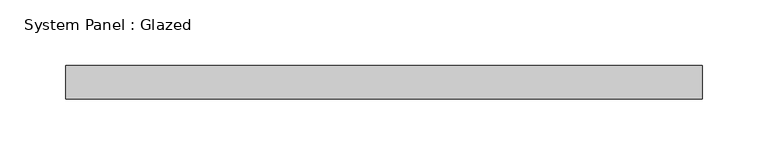
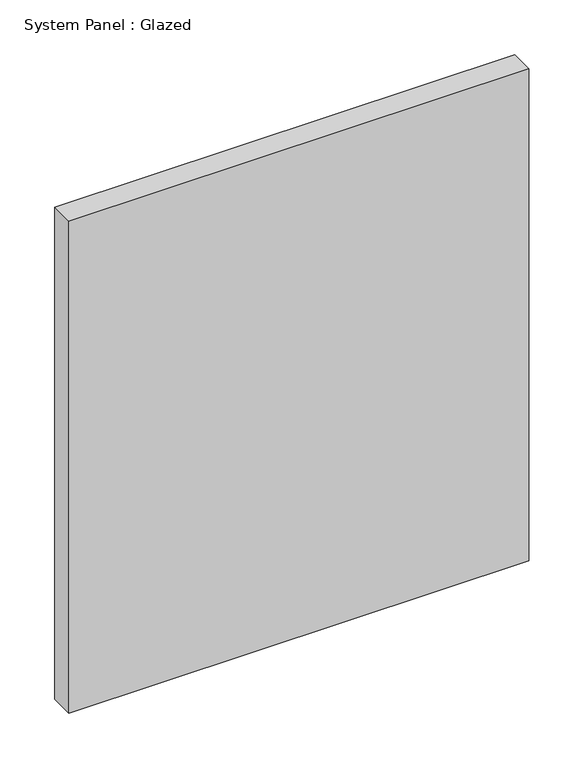
"""IFC4 building model written with IfcOpenShell, lengths in millimetres: plate geometry, System Panel : Glazed."""

from ifc_helpers import new_model, si_unit, origin, origin_with_axes, place, context, project, spatial, polyline, outline, extrude, source, transform, mapped, element, save


def system_panel_glazed_07c93182(model_context):
    return source(origin(), model_context, "Body", "SweptSolid", [
        extrude(outline(polyline([(241.3, 19.05), (-241.3, 19.05), (-241.3, 44.45), (241.3, 44.45), (241.3, 19.05)])), origin_with_axes(), (0.0, 0.0, 1.0), 546.1),
    ])


if __name__ == "__main__":
    model = new_model("IFC4")
    model_context = context("Model", 3, world=origin())
    ifc_project = project(units=[si_unit("LENGTHUNIT", "METRE", prefix="MILLI")], contexts=[model_context])
    site = spatial("IfcSite", under=ifc_project)
    building = spatial("IfcBuilding", under=site)
    placement = place(None, origin())
    system_panel_glazed_shape = system_panel_glazed_07c93182(model_context)
    element("IfcPlate", 1, ObjectType="System Panel : Glazed", at=placement, inside=building, context=model_context, shape_type="MappedRepresentation", body=[
        mapped(system_panel_glazed_shape, transform((0.0, 0.0, 0.0), x_axis=(1.0, 0.0, 0.0), y_axis=(0.0, 1.0, 0.0), z_axis=(0.0, 0.0, 1.0))),
    ])
    save(model, "model.ifc")

# Revit data of these elements
# Type "System Panel : Glazed"
#   Construction Type Id = "GSP4R"
#   Analytic Construction = "1/8 in Pilkington single glazing"
#   Visual Light Transmittance = 0.9
#   Solar Heat Gain Coefficient = 0.86
#   Heat Transfer Coefficient (U) = 1.18115 BTU/(h·ft²·°F)
#   Define Thermal Properties by = 1
# Element 1 (IfcPlate, "System Panel : Glazed")
#   Materials on its faces: "Glass"
# Materials
#   "Glass": class "Glass", colour RGB 0 128 192, transparency 0.75, Description = "Soda Lime Glass", Cost = 0
